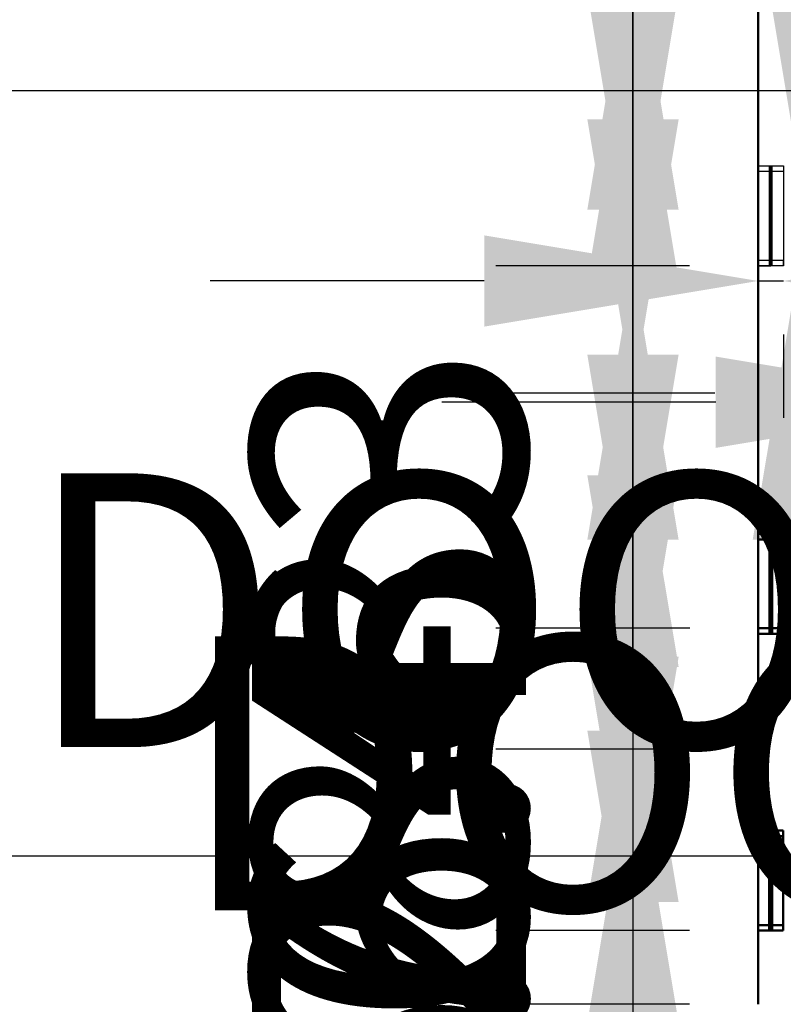
# Model space of a CAD drawing. Units: metres. Extents: x 782 to 1487, y 1262 to 7446.
# Tile 13 of 25: x 821.225 to 828.192, y 1293.067 to 1302.058. Entities that reach past the tile are written whole.
import ezdxf

# ---------------------------------------------------------------- set-up
doc = ezdxf.new("R2010")
doc.units = ezdxf.units.M
for name, color, linetype, lineweight in [('A-ANNO-DIMS', 2, 'Continuous', 18), ('A-GLAZ', 4, 'Continuous', 25), ('A-WALL', 7, 'Continuous', 50)]:
    doc.layers.add(name, color=color, linetype=linetype, lineweight=lineweight)
doc.styles.get("Standard").update_dxf_attribs({"font": 'arial.ttf'})
doc.dimstyles.new('ISO-25', dxfattribs={"dimtxt": 2.5, "dimasz": 2.5, "dimexe": 1.25, "dimexo": 0.625, "dimtad": 1, "dimtxsty": 'Standard', "dimcen": 2.5, "dimadec": 0, "dimazin": 0, "dimtfac": 1, "dimtmove": 0, "dimatfit": 3, "dimfxl": 1, "dimarcsym": 0})

# ---------------------------------------------------------------- blocks, each defined once
blk = doc.blocks.new('WIN-900')
for p, q in [((0.0001, -0.0002), (0.0001, 0.9138)), ((0.0001, 0.9138), (0.2301, 0.9138)), ((0.1024, -0.0002), (0.1024, 0.9138)), ((0.1151, -0.0002), (0.1151, 0.9138)), ((0.1278, -0.0002), (0.1278, 0.9138)), ((0.2301, 0.9138), (0.2301, -0.0002)), ((0.2301, 0.9138), (0.2301, 0.863)), ((0.2301, 0.863), (0.0001, 0.863)), ((0.2301, 0.0506), (0.0001, 0.0506)), ((0.2301, -0.0002), (0.2301, 0.0506)), ((0.2301, -0.0002), (0.0001, -0.0002)), ((0.0001, -0.0002), (0.1151, -0.0002))]:
    blk.add_line(p, q)
blk = doc.blocks.new('*D20')
at = {"layer": 'A-ANNO-DIMS', "color": 0, "lineweight": -2, "transparency": 16777216}
for p, q in [((831.0564, 1302.0877), (831.0564, 1337.6778)), ((831.0564, 1298.6982), (831.0564, 1299.5877)), ((831.548, 1299.5877), (832.3064, 1299.5877)), ((831.548, 1298.6982), (832.3064, 1298.6982)), ((831.0564, 1296.1982), (831.0564, 1293.6982))]:
    blk.add_line(p, q, dxfattribs=at)
at = {"layer": 'A-ANNO-DIMS', "color": 0, "transparency": 16777216}
for points in [[(830.6398, 1302.0877), (831.4731, 1302.0877), (831.0564, 1299.5877)], [(830.6398, 1296.1982), (831.4731, 1296.1982), (831.0564, 1298.6982)]]:
    blk.add_solid(points, dxfattribs=at)
at = {"layer": 'Defpoints', "color": 0, "transparency": 16777216}
for p in [(830.923, 1299.5877), (831.0564, 1299.5877), (830.923, 1298.6982)]:
    blk.add_point(p, dxfattribs=at)
at = {"layer": 'A-ANNO-DIMS', "color": 0, "transparency": 16777216, "insert": (829.138, 1321.1327), "char_height": 2.5, "attachment_point": 5, "rotation": 90}
blk.add_mtext('DOOR D1 0.89 TYP.', dxfattribs=at)
blk = doc.blocks.new('*D21')
at = {"layer": 'A-ANNO-DIMS', "color": 0, "lineweight": -2, "transparency": 16777216}
for p, q in [((827.5763, 1298.5648), (825.0763, 1298.5648)), ((830.0763, 1298.5648), (830.923, 1298.5648)), ((833.423, 1298.5648), (852.2549, 1298.5648)), ((830.0763, 1298.0732), (830.0763, 1297.3148)), ((830.923, 1298.0732), (830.923, 1297.3148))]:
    blk.add_line(p, q, dxfattribs=at)
at = {"layer": 'A-ANNO-DIMS', "color": 0, "transparency": 16777216}
for points in [[(827.5763, 1298.9815), (827.5763, 1298.1481), (830.0763, 1298.5648)], [(833.423, 1298.9815), (833.423, 1298.1481), (830.923, 1298.5648)]]:
    blk.add_solid(points, dxfattribs=at)
at = {"layer": 'Defpoints', "color": 0, "transparency": 16777216}
for p in [(830.0763, 1298.6982), (830.923, 1298.6982), (830.923, 1298.5648)]:
    blk.add_point(p, dxfattribs=at)
at = {"layer": 'A-ANNO-DIMS', "color": 0, "transparency": 16777216, "insert": (844.0889, 1300.4662), "char_height": 2.5, "attachment_point": 5}
blk.add_mtext('0.85 TYP.', dxfattribs=at)
blk = doc.blocks.new('*D22')
at = {"layer": 'A-ANNO-DIMS', "color": 0, "lineweight": -2, "transparency": 16777216}
for p, q in [((812.7897, 1292.934), (810.2897, 1292.934)), ((815.2897, 1292.934), (816.1792, 1292.934)), ((818.6792, 1292.934), (848.8344, 1292.934)), ((815.2897, 1292.4424), (815.2897, 1291.684)), ((816.1792, 1292.4424), (816.1792, 1291.684))]:
    blk.add_line(p, q, dxfattribs=at)
at = {"layer": 'A-ANNO-DIMS', "color": 0, "transparency": 16777216}
for points in [[(812.7897, 1293.3507), (812.7897, 1292.5173), (815.2897, 1292.934)], [(818.6792, 1293.3507), (818.6792, 1292.5173), (816.1792, 1292.934)]]:
    blk.add_solid(points, dxfattribs=at)
at = {"layer": 'Defpoints', "color": 0, "transparency": 16777216}
for p in [(815.2897, 1293.0674), (816.1792, 1293.0674), (816.1792, 1292.934)]:
    blk.add_point(p, dxfattribs=at)
at = {"layer": 'A-ANNO-DIMS', "color": 0, "transparency": 16777216, "insert": (835.0068, 1294.8525), "char_height": 2.5, "attachment_point": 5}
blk.add_mtext('DOOR 0.89 TYP.', dxfattribs=at)
blk = doc.blocks.new('*D24')
at = {"layer": 'A-ANNO-DIMS', "color": 0, "lineweight": -2, "transparency": 16777216}
for p, q in [((811.2086, 1294.4231), (808.7086, 1294.4231)), ((813.7086, 1294.4231), (814.5592, 1294.4231)), ((817.0592, 1294.4231), (852.6493, 1294.4231)), ((813.7086, 1293.9257), (813.7086, 1293.1731)), ((814.5592, 1293.9257), (814.5592, 1293.1731))]:
    blk.add_line(p, q, dxfattribs=at)
at = {"layer": 'A-ANNO-DIMS', "color": 0, "transparency": 16777216}
for points in [[(811.2086, 1294.8398), (811.2086, 1294.0065), (813.7086, 1294.4231)], [(817.0592, 1294.8398), (817.0592, 1294.0065), (814.5592, 1294.4231)]]:
    blk.add_solid(points, dxfattribs=at)
at = {"layer": 'Defpoints', "color": 0, "transparency": 16777216}
for p in [(813.7086, 1294.5507), (814.5592, 1294.5507), (814.5592, 1294.4231)]:
    blk.add_point(p, dxfattribs=at)
at = {"layer": 'A-ANNO-DIMS', "color": 0, "transparency": 16777216, "insert": (836.1042, 1296.3416), "char_height": 2.5, "attachment_point": 5}
blk.add_mtext('DOOR D2 0.85 TYP.', dxfattribs=at)
blk = doc.blocks.new('*D26')
at = {"layer": 'A-ANNO-DIMS', "color": 0, "lineweight": -2, "transparency": 16777216}
for p, q in [((828.3302, 1303.2228), (828.3302, 1342.7181)), ((828.3302, 1299.8088), (828.3302, 1300.7228)), ((828.8181, 1300.7228), (829.5802, 1300.7228)), ((828.8181, 1299.8088), (829.5802, 1299.8088)), ((828.3302, 1297.3088), (828.3302, 1294.8088))]:
    blk.add_line(p, q, dxfattribs=at)
at = {"layer": 'A-ANNO-DIMS', "color": 0, "transparency": 16777216}
for points in [[(827.9135, 1303.2228), (828.7468, 1303.2228), (828.3302, 1300.7228)], [(827.9135, 1297.3088), (828.7468, 1297.3088), (828.3302, 1299.8088)]]:
    blk.add_solid(points, dxfattribs=at)
at = {"layer": 'Defpoints', "color": 0, "transparency": 16777216}
for p in [(828.1931, 1300.7228), (828.3302, 1300.7228), (828.1931, 1299.8088)]:
    blk.add_point(p, dxfattribs=at)
at = {"layer": 'A-ANNO-DIMS', "color": 0, "transparency": 16777216, "insert": (826.4117, 1324.2204), "char_height": 2.5, "attachment_point": 5, "rotation": 90}
blk.add_mtext('WINDOW W 0.91 TYP.', dxfattribs=at)
blk = doc.blocks.new('*D27')
at = {"layer": 'A-ANNO-DIMS', "color": 0, "lineweight": -2, "transparency": 16777216}
for p, q in [((825.4631, 1299.6717), (822.9631, 1299.6717)), ((827.9631, 1299.6717), (828.1931, 1299.6717)), ((830.6931, 1299.6717), (849.5249, 1299.6717)), ((827.9631, 1299.1838), (827.9631, 1298.4217)), ((828.1931, 1299.1838), (828.1931, 1298.4217))]:
    blk.add_line(p, q, dxfattribs=at)
at = {"layer": 'A-ANNO-DIMS', "color": 0, "transparency": 16777216}
for points in [[(825.4631, 1300.0884), (825.4631, 1299.2551), (827.9631, 1299.6717)], [(830.6931, 1300.0884), (830.6931, 1299.2551), (828.1931, 1299.6717)]]:
    blk.add_solid(points, dxfattribs=at)
at = {"layer": 'Defpoints', "color": 0, "transparency": 16777216}
for p in [(827.9631, 1299.8088), (828.1931, 1299.8088), (828.1931, 1299.6717)]:
    blk.add_point(p, dxfattribs=at)
at = {"layer": 'A-ANNO-DIMS', "color": 0, "transparency": 16777216, "insert": (841.359, 1301.574), "char_height": 2.5, "attachment_point": 5}
blk.add_mtext('0.23 TYP.', dxfattribs=at)
blk = doc.blocks.new('*D28')
at = {"layer": 'A-ANNO-DIMS', "color": 0, "lineweight": -2, "transparency": 16777216}
for p, q in [((832.5503, 1308.2809), (832.5503, 1349.7185)), ((832.5503, 1304.8669), (832.5503, 1305.7809)), ((833.0382, 1305.7809), (833.8003, 1305.7809)), ((833.0382, 1304.8669), (833.8003, 1304.8669)), ((832.5503, 1302.3669), (832.5503, 1299.8669))]:
    blk.add_line(p, q, dxfattribs=at)
at = {"layer": 'A-ANNO-DIMS', "color": 0, "transparency": 16777216}
for points in [[(832.1336, 1308.2809), (832.967, 1308.2809), (832.5503, 1305.7809)], [(832.1336, 1302.3669), (832.967, 1302.3669), (832.5503, 1304.8669)]]:
    blk.add_solid(points, dxfattribs=at)
at = {"layer": 'Defpoints', "color": 0, "transparency": 16777216}
for p in [(832.4132, 1305.7809), (832.5503, 1305.7809), (832.4132, 1304.8669)]:
    blk.add_point(p, dxfattribs=at)
at = {"layer": 'A-ANNO-DIMS', "color": 0, "transparency": 16777216, "insert": (830.6318, 1330.2497), "char_height": 2.5, "attachment_point": 5, "rotation": 90}
blk.add_mtext('WINDOW W1 0.91 TYP.', dxfattribs=at)
blk = doc.blocks.new('*D30')
at = {"layer": 'A-ANNO-DIMS', "color": 0, "lineweight": -2, "transparency": 16777216}
for p, q in [((792.059, 1301.4107), (789.559, 1301.4107)), ((794.559, 1301.4107), (794.9459, 1301.4107)), ((797.4459, 1301.4107), (832.3538, 1301.4107)), ((794.559, 1300.8437), (794.559, 1300.1607)), ((794.9459, 1300.8437), (794.9459, 1300.1607))]:
    blk.add_line(p, q, dxfattribs=at)
at = {"layer": 'A-ANNO-DIMS', "color": 0, "transparency": 16777216}
for points in [[(792.059, 1301.8274), (792.059, 1300.994), (794.559, 1301.4107)], [(797.4459, 1301.8274), (797.4459, 1300.994), (794.9459, 1301.4107)]]:
    blk.add_solid(points, dxfattribs=at)
at = {"layer": 'Defpoints', "color": 0, "transparency": 16777216}
for p in [(794.559, 1301.4687), (794.9459, 1301.4687), (794.9459, 1301.4107)]:
    blk.add_point(p, dxfattribs=at)
at = {"layer": 'A-ANNO-DIMS', "color": 0, "transparency": 16777216, "insert": (816.1499, 1303.33), "char_height": 2.5, "attachment_point": 5}
blk.add_mtext('COLUMN 0.39 TYP.', dxfattribs=at)
blk = doc.blocks.new('*D77')
at = {"layer": 'A-ANNO-DIMS', "color": 0, "lineweight": -2, "transparency": 16777216}
for p, q in [((826.8209, 1309.8274), (826.8209, 1312.3274)), ((827.3375, 1307.3274), (825.5709, 1307.3274)), ((826.8209, 1307.3274), (826.8209, 1304.6974)), ((827.5675, 1304.6974), (825.5709, 1304.6974)), ((826.8209, 1302.1974), (826.8209, 1291.9109))]:
    blk.add_line(p, q, dxfattribs=at)
at = {"layer": 'A-ANNO-DIMS', "color": 0, "transparency": 16777216}
for points in [[(826.4043, 1309.8274), (827.2376, 1309.8274), (826.8209, 1307.3274)], [(826.4043, 1302.1974), (827.2376, 1302.1974), (826.8209, 1304.6974)]]:
    blk.add_solid(points, dxfattribs=at)
at = {"layer": 'Defpoints', "color": 0, "transparency": 16777216}
for p in [(827.9625, 1307.3274), (826.8209, 1304.6974), (828.1925, 1304.6974)]:
    blk.add_point(p, dxfattribs=at)
at = {"layer": 'A-ANNO-DIMS', "color": 0, "transparency": 16777216, "insert": (824.9186, 1295.8042), "char_height": 2.5, "attachment_point": 5, "rotation": 90}
blk.add_mtext('2.63', dxfattribs=at)
blk = doc.blocks.new('*D78')
at = {"layer": 'A-ANNO-DIMS', "color": 0, "lineweight": -2, "transparency": 16777216}
for p, q in [((826.8209, 1307.1974), (826.8209, 1309.6974)), ((827.5675, 1304.6974), (825.5709, 1304.6974)), ((826.8209, 1304.6974), (826.8209, 1302.8221)), ((827.3359, 1302.8221), (825.5709, 1302.8221)), ((826.8209, 1300.3221), (826.8209, 1290.3084))]:
    blk.add_line(p, q, dxfattribs=at)
at = {"layer": 'A-ANNO-DIMS', "color": 0, "transparency": 16777216}
for points in [[(826.4043, 1307.1974), (827.2376, 1307.1974), (826.8209, 1304.6974)], [(826.4043, 1300.3221), (827.2376, 1300.3221), (826.8209, 1302.8221)]]:
    blk.add_solid(points, dxfattribs=at)
at = {"layer": 'Defpoints', "color": 0, "transparency": 16777216}
for p in [(828.1925, 1304.6974), (826.8209, 1302.8221), (827.9609, 1302.8221)]:
    blk.add_point(p, dxfattribs=at)
at = {"layer": 'A-ANNO-DIMS', "color": 0, "transparency": 16777216, "insert": (824.9195, 1294.0652), "char_height": 2.5, "attachment_point": 5, "rotation": 90}
blk.add_mtext('1.88', dxfattribs=at)
blk = doc.blocks.new('*D79')
at = {"layer": 'A-ANNO-DIMS', "color": 0, "lineweight": -2, "transparency": 16777216}
for p, q in [((826.8209, 1305.3221), (826.8209, 1307.8221)), ((827.3359, 1302.8221), (825.5709, 1302.8221)), ((826.8209, 1302.8221), (826.8209, 1302.1774)), ((827.5675, 1302.1774), (825.5709, 1302.1774)), ((826.8209, 1299.6774), (826.8209, 1289.4438))]:
    blk.add_line(p, q, dxfattribs=at)
at = {"layer": 'A-ANNO-DIMS', "color": 0, "transparency": 16777216}
for points in [[(826.4043, 1305.3221), (827.2376, 1305.3221), (826.8209, 1302.8221)], [(826.4043, 1299.6774), (827.2376, 1299.6774), (826.8209, 1302.1774)]]:
    blk.add_solid(points, dxfattribs=at)
at = {"layer": 'Defpoints', "color": 0, "transparency": 16777216}
for p in [(827.9609, 1302.8221), (826.8209, 1302.1774), (828.1925, 1302.1774)]:
    blk.add_point(p, dxfattribs=at)
at = {"layer": 'A-ANNO-DIMS', "color": 0, "transparency": 16777216, "insert": (824.9195, 1293.3106), "char_height": 2.5, "attachment_point": 5, "rotation": 90}
blk.add_mtext('0.64', dxfattribs=at)
blk = doc.blocks.new('*D80')
at = {"layer": 'A-ANNO-DIMS', "color": 0, "lineweight": -2, "transparency": 16777216}
for p, q in [((826.8209, 1304.6774), (826.8209, 1307.1774)), ((827.5675, 1302.1774), (825.5709, 1302.1774)), ((826.8209, 1302.1774), (826.8209, 1299.8088)), ((827.3381, 1299.8088), (825.5709, 1299.8088)), ((826.8209, 1297.3088), (826.8209, 1287.0223))]:
    blk.add_line(p, q, dxfattribs=at)
at = {"layer": 'A-ANNO-DIMS', "color": 0, "transparency": 16777216}
for points in [[(826.4043, 1304.6774), (827.2376, 1304.6774), (826.8209, 1302.1774)], [(826.4043, 1297.3088), (827.2376, 1297.3088), (826.8209, 1299.8088)]]:
    blk.add_solid(points, dxfattribs=at)
at = {"layer": 'Defpoints', "color": 0, "transparency": 16777216}
for p in [(828.1925, 1302.1774), (826.8209, 1299.8088), (827.9631, 1299.8088)]:
    blk.add_point(p, dxfattribs=at)
at = {"layer": 'A-ANNO-DIMS', "color": 0, "transparency": 16777216, "insert": (824.9186, 1290.9156), "char_height": 2.5, "attachment_point": 5, "rotation": 90}
blk.add_mtext('2.37', dxfattribs=at)
blk = doc.blocks.new('*D81')
at = {"layer": 'A-ANNO-DIMS', "color": 0, "lineweight": -2, "transparency": 16777216}
for p, q in [((826.8209, 1302.3088), (826.8209, 1304.8088)), ((827.3381, 1299.8088), (825.5709, 1299.8088)), ((826.8209, 1299.8088), (826.8209, 1298.6474)), ((827.5675, 1298.6474), (825.5709, 1298.6474)), ((826.8209, 1296.1474), (826.8209, 1286.1406))]:
    blk.add_line(p, q, dxfattribs=at)
at = {"layer": 'A-ANNO-DIMS', "color": 0, "transparency": 16777216}
for points in [[(826.4043, 1302.3088), (827.2376, 1302.3088), (826.8209, 1299.8088)], [(826.4043, 1296.1474), (827.2376, 1296.1474), (826.8209, 1298.6474)]]:
    blk.add_solid(points, dxfattribs=at)
at = {"layer": 'Defpoints', "color": 0, "transparency": 16777216}
for p in [(827.9631, 1299.8088), (826.8209, 1298.6474), (828.1925, 1298.6474)]:
    blk.add_point(p, dxfattribs=at)
at = {"layer": 'A-ANNO-DIMS', "color": 0, "transparency": 16777216, "insert": (824.9195, 1289.894), "char_height": 2.5, "attachment_point": 5, "rotation": 90}
blk.add_mtext('1.16', dxfattribs=at)
blk = doc.blocks.new('*D82')
at = {"layer": 'A-ANNO-DIMS', "color": 0, "lineweight": -2, "transparency": 16777216}
for p, q in [((826.8209, 1301.1474), (826.8209, 1303.6474)), ((827.5675, 1298.6474), (825.5709, 1298.6474)), ((826.8209, 1298.6474), (826.8209, 1296.5004)), ((827.3391, 1296.5004), (825.5709, 1296.5004)), ((826.8209, 1294.0004), (826.8209, 1281.7715))]:
    blk.add_line(p, q, dxfattribs=at)
at = {"layer": 'A-ANNO-DIMS', "color": 0, "transparency": 16777216}
for points in [[(826.4043, 1301.1474), (827.2376, 1301.1474), (826.8209, 1298.6474)], [(826.4043, 1294.0004), (827.2376, 1294.0004), (826.8209, 1296.5004)]]:
    blk.add_solid(points, dxfattribs=at)
at = {"layer": 'Defpoints', "color": 0, "transparency": 16777216}
for p in [(828.1925, 1298.6474), (826.8209, 1296.5004), (827.9641, 1296.5004)]:
    blk.add_point(p, dxfattribs=at)
at = {"layer": 'A-ANNO-DIMS', "color": 0, "transparency": 16777216, "insert": (824.9408, 1286.636), "char_height": 2.5, "attachment_point": 5, "rotation": 90}
blk.add_mtext('2.147', dxfattribs=at)
blk = doc.blocks.new('*D83')
at = {"layer": 'A-ANNO-DIMS', "color": 0, "lineweight": -2, "transparency": 16777216}
for p, q in [((826.8209, 1299.0004), (826.8209, 1301.5004)), ((827.3391, 1296.5004), (825.5709, 1296.5004)), ((826.8209, 1296.5004), (826.8209, 1295.3974)), ((827.5675, 1295.3974), (825.5709, 1295.3974)), ((826.8209, 1292.8974), (826.8209, 1280.9465))]:
    blk.add_line(p, q, dxfattribs=at)
at = {"layer": 'A-ANNO-DIMS', "color": 0, "transparency": 16777216}
for points in [[(826.4043, 1299.0004), (827.2376, 1299.0004), (826.8209, 1296.5004)], [(826.4043, 1292.8974), (827.2376, 1292.8974), (826.8209, 1295.3974)]]:
    blk.add_solid(points, dxfattribs=at)
at = {"layer": 'Defpoints', "color": 0, "transparency": 16777216}
for p in [(827.9641, 1296.5004), (826.8209, 1295.3974), (828.1925, 1295.3974)]:
    blk.add_point(p, dxfattribs=at)
at = {"layer": 'A-ANNO-DIMS', "color": 0, "transparency": 16777216, "insert": (824.9186, 1285.672), "char_height": 2.5, "attachment_point": 5, "rotation": 90}
blk.add_mtext('1.103', dxfattribs=at)
blk = doc.blocks.new('*D84')
at = {"layer": 'A-ANNO-DIMS', "color": 0, "lineweight": -2, "transparency": 16777216}
for p, q in [((826.8209, 1297.8974), (826.8209, 1300.3974)), ((827.5675, 1295.3974), (825.5709, 1295.3974)), ((826.8209, 1295.3974), (826.8209, 1293.7402)), ((827.3372, 1293.7402), (825.5709, 1293.7402)), ((826.8209, 1291.2402), (826.8209, 1281.2334))]:
    blk.add_line(p, q, dxfattribs=at)
at = {"layer": 'A-ANNO-DIMS', "color": 0, "transparency": 16777216}
for points in [[(826.4043, 1297.8974), (827.2376, 1297.8974), (826.8209, 1295.3974)], [(826.4043, 1291.2402), (827.2376, 1291.2402), (826.8209, 1293.7402)]]:
    blk.add_solid(points, dxfattribs=at)
at = {"layer": 'Defpoints', "color": 0, "transparency": 16777216}
for p in [(828.1925, 1295.3974), (826.8209, 1293.7402), (827.9622, 1293.7402)]:
    blk.add_point(p, dxfattribs=at)
at = {"layer": 'A-ANNO-DIMS', "color": 0, "transparency": 16777216, "insert": (824.9195, 1284.9868), "char_height": 2.5, "attachment_point": 5, "rotation": 90}
blk.add_mtext('1.66', dxfattribs=at)
blk = doc.blocks.new('*D85')
at = {"layer": 'A-ANNO-DIMS', "color": 0, "lineweight": -2, "transparency": 16777216}
for p, q in [((826.8209, 1296.2402), (826.8209, 1298.7402)), ((827.3372, 1293.7402), (825.5709, 1293.7402)), ((826.8209, 1293.7402), (826.8209, 1293.0674)), ((827.3375, 1293.0674), (825.5709, 1293.0674)), ((826.8209, 1290.5674), (826.8209, 1280.3236))]:
    blk.add_line(p, q, dxfattribs=at)
at = {"layer": 'A-ANNO-DIMS', "color": 0, "transparency": 16777216}
for points in [[(826.4043, 1296.2402), (827.2376, 1296.2402), (826.8209, 1293.7402)], [(826.4043, 1290.5674), (827.2376, 1290.5674), (826.8209, 1293.0674)]]:
    blk.add_solid(points, dxfattribs=at)
at = {"layer": 'Defpoints', "color": 0, "transparency": 16777216}
for p in [(827.9622, 1293.7402), (826.8209, 1293.0674), (827.9625, 1293.0674)]:
    blk.add_point(p, dxfattribs=at)
at = {"layer": 'A-ANNO-DIMS', "color": 0, "transparency": 16777216, "insert": (824.9195, 1284.1955), "char_height": 2.5, "attachment_point": 5, "rotation": 90}
blk.add_mtext('0.67', dxfattribs=at)
blk = doc.blocks.new('*D86')
at = {"layer": 'A-ANNO-DIMS', "color": 0, "lineweight": -2, "transparency": 16777216}
for p, q in [((826.8209, 1295.5674), (826.8209, 1298.0674)), ((827.3375, 1293.0674), (825.5709, 1293.0674)), ((826.8209, 1293.0674), (826.8209, 1290.3053)), ((827.3375, 1290.3053), (825.5709, 1290.3053)), ((826.8209, 1287.8053), (826.8209, 1275.602))]:
    blk.add_line(p, q, dxfattribs=at)
at = {"layer": 'A-ANNO-DIMS', "color": 0, "transparency": 16777216}
for points in [[(826.4043, 1295.5674), (827.2376, 1295.5674), (826.8209, 1293.0674)], [(826.4043, 1287.8053), (827.2376, 1287.8053), (826.8209, 1290.3053)]]:
    blk.add_solid(points, dxfattribs=at)
at = {"layer": 'Defpoints', "color": 0, "transparency": 16777216}
for p in [(827.9625, 1293.0674), (826.8209, 1290.3053), (827.9625, 1290.3053)]:
    blk.add_point(p, dxfattribs=at)
at = {"layer": 'A-ANNO-DIMS', "color": 0, "transparency": 16777216, "insert": (824.9195, 1280.4536), "char_height": 2.5, "attachment_point": 5, "rotation": 90}
blk.add_mtext('2.762', dxfattribs=at)

msp = doc.modelspace()

# ---------------------------------------------------------------- linework, layer by layer
at = {"layer": 'A-WALL'}
for p, q in [((827.9625, 1298.6474), (827.9625, 1302.1774)), ((827.9625, 1295.3974), (827.9625, 1298.6474)), ((827.9641, 1296.4496), (827.9641, 1297.3636)), ((827.9641, 1297.3636), (828.1941, 1297.3636)), ((828.0664, 1296.4496), (828.0664, 1297.3636)), ((828.0791, 1296.4496), (828.0791, 1297.3636)), ((828.0918, 1296.4496), (828.0918, 1297.3636)), ((828.1941, 1297.3128), (827.9641, 1297.3128)), ((828.1941, 1296.5004), (827.9641, 1296.5004)), ((828.1941, 1296.4496), (827.9641, 1296.4496)), ((827.9641, 1296.4496), (828.0791, 1296.4496)), ((827.9625, 1295.3974), (827.9625, 1293.0674)), ((827.9622, 1293.7402), (827.9622, 1294.6542)), ((827.9622, 1294.6542), (828.1922, 1294.6542)), ((828.1922, 1294.6034), (827.9622, 1294.6034)), ((828.0645, 1293.7402), (828.0645, 1294.6542)), ((828.0772, 1293.7402), (828.0772, 1294.6542)), ((828.0899, 1293.7402), (828.0899, 1294.6542)), ((828.1922, 1294.6542), (828.1922, 1293.7402)), ((828.1922, 1294.6542), (828.1922, 1294.6034)), ((828.1922, 1293.791), (827.9622, 1293.791)), ((828.1922, 1293.7402), (828.1922, 1293.791)), ((828.1922, 1293.7402), (827.9622, 1293.7402)), ((827.9622, 1293.7402), (828.0772, 1293.7402))]:
    msp.add_line(p, q, dxfattribs=at)

# ---------------------------------------------------------------- block references
at = {"layer": 'A-GLAZ'}
msp.add_blockref('WIN-900', (827.963, 1299.809), dxfattribs=at)

# ---------------------------------------------------------------- dimensions: what is measured, and where the dimension line sits
at = {"layer": 'A-ANNO-DIMS'}
for base, p1, p2, text, picture, middle in [((832.5503, 1305.7809), (832.4132, 1304.8669), (832.4132, 1305.7809), 'WINDOW W1 <> TYP.', '*D28', (830.6318, 1330.2497)), ((828.3302, 1300.7228), (828.1931, 1299.8088), (828.1931, 1300.7228), 'WINDOW W <> TYP.', '*D26', (826.4117, 1324.2204)), ((831.0564, 1299.5877), (830.923, 1298.6982), (830.923, 1299.5877), 'DOOR D1 <> TYP.', '*D20', (829.138, 1321.1327))]:
    dim = msp.add_linear_dim(base=base, p1=p1, p2=p2, angle=90, text=text, dimstyle='ISO-25', override={"dimdec": 2, "dimlfac": 1, "dimrnd": 0, "dimzin": 0, "dimdsep": 46, "dimlunit": 2}, dxfattribs=at)
    dim.commit()
    dim.dimension.update_dxf_attribs({"geometry": picture, "text_midpoint": middle})
for base, p1, p2, override, picture, middle in [((826.8209, 1304.6974), (827.9625, 1307.3274), (828.1925, 1304.6974), {"dimdec": 2, "dimlfac": 1, "dimrnd": 0, "dimzin": 0, "dimdsep": 46, "dimlunit": 2}, '*D77', (824.9186, 1295.8042)), ((826.8209, 1302.8221), (828.1925, 1304.6974), (827.9609, 1302.8221), {"dimdec": 2, "dimlfac": 1, "dimrnd": 0, "dimzin": 0, "dimdsep": 46, "dimlunit": 2}, '*D78', (824.9195, 1294.0652)), ((826.8209, 1302.1774), (827.9609, 1302.8221), (828.1925, 1302.1774), {"dimdec": 2, "dimlfac": 1, "dimrnd": 0, "dimzin": 0, "dimdsep": 46, "dimlunit": 2}, '*D79', (824.9195, 1293.3106)), ((826.8209, 1299.8088), (828.1925, 1302.1774), (827.9631, 1299.8088), {"dimdec": 2, "dimlfac": 1, "dimrnd": 0, "dimzin": 0, "dimdsep": 46, "dimlunit": 2}, '*D80', (824.9186, 1290.9156)), ((826.8209, 1298.6474), (827.9631, 1299.8088), (828.1925, 1298.6474), {"dimdec": 2, "dimlfac": 1, "dimrnd": 0, "dimzin": 0, "dimdsep": 46, "dimlunit": 2}, '*D81', (824.9195, 1289.894)), ((826.8209, 1296.5004), (828.1925, 1298.6474), (827.9641, 1296.5004), {"dimdec": 3, "dimlfac": 1, "dimrnd": 0, "dimzin": 0, "dimdsep": 46, "dimlunit": 2}, '*D82', (824.9408, 1286.636)), ((826.8209, 1295.3974), (827.9641, 1296.5004), (828.1925, 1295.3974), {"dimdec": 3, "dimlfac": 1, "dimrnd": 0, "dimzin": 0, "dimdsep": 46, "dimlunit": 2}, '*D83', (824.9186, 1285.672)), ((826.8209, 1293.7402), (828.1925, 1295.3974), (827.9622, 1293.7402), {"dimdec": 2, "dimlfac": 1, "dimrnd": 0, "dimzin": 0, "dimdsep": 46, "dimlunit": 2}, '*D84', (824.9195, 1284.9868)), ((826.8209, 1293.0674), (827.9622, 1293.7402), (827.9625, 1293.0674), {"dimdec": 2, "dimlfac": 1, "dimrnd": 0, "dimzin": 0, "dimdsep": 46, "dimlunit": 2}, '*D85', (824.9195, 1284.1955)), ((826.8209, 1290.3053), (827.9625, 1293.0674), (827.9625, 1290.3053), {"dimdec": 3, "dimlfac": 1, "dimrnd": 0, "dimzin": 0, "dimdsep": 46, "dimlunit": 2}, '*D86', (824.9195, 1280.4536))]:
    dim = msp.add_linear_dim(base=base, p1=p1, p2=p2, angle=90, dimstyle='ISO-25', override=override, dxfattribs=at)
    dim.commit()
    dim.dimension.update_dxf_attribs({"geometry": picture, "text_midpoint": middle})
for base, p1, p2, text, picture, middle in [((794.9459, 1301.4107), (794.559, 1301.4687), (794.9459, 1301.4687), 'COLUMN <> TYP.', '*D30', (816.1499, 1303.33)), ((828.1931, 1299.6717), (827.9631, 1299.8088), (828.1931, 1299.8088), '<> TYP.', '*D27', (841.359, 1301.574)), ((814.5592, 1294.4231), (813.7086, 1294.5507), (814.5592, 1294.5507), 'DOOR D2 <> TYP.', '*D24', (836.1042, 1296.3416)), ((830.923, 1298.5648), (830.0763, 1298.6982), (830.923, 1298.6982), '<> TYP.', '*D21', (844.0889, 1300.4662)), ((816.1792, 1292.934), (815.2897, 1293.0674), (816.1792, 1293.0674), 'DOOR <> TYP.', '*D22', (835.0068, 1294.8525))]:
    dim = msp.add_linear_dim(base=base, p1=p1, p2=p2, text=text, dimstyle='ISO-25', override={"dimdec": 2, "dimlfac": 1, "dimrnd": 0, "dimzin": 0, "dimdsep": 46, "dimlunit": 2}, dxfattribs=at)
    dim.commit()
    dim.dimension.update_dxf_attribs({"geometry": picture, "text_midpoint": middle})

doc.saveas('drawing.dxf')
